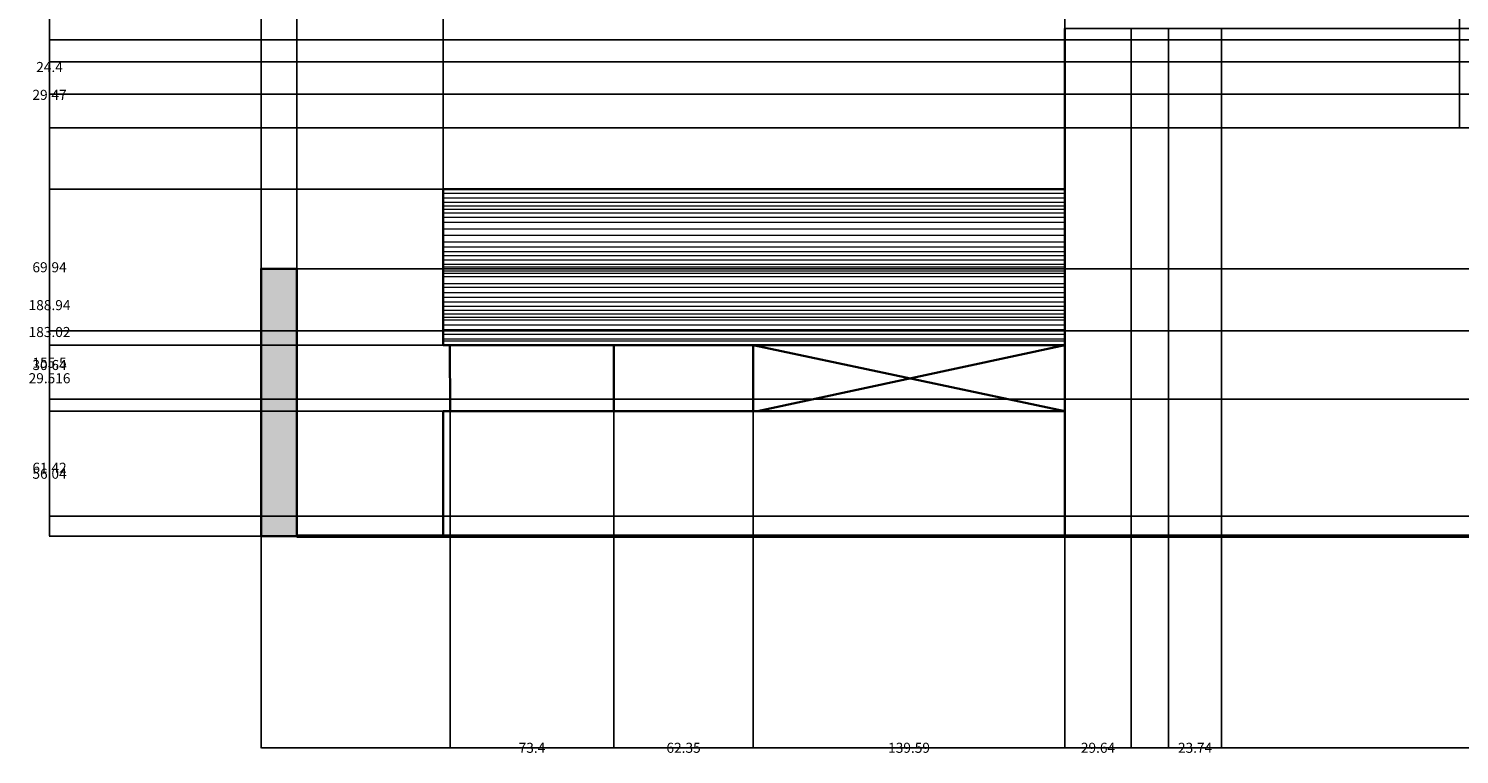
# Model space of a CAD drawing. Units: inches. Extents: x -1308 to 780, y 304 to 1023.
# Tile 1 of 7: x -1308 to -667, y 304 to 629. Entities that reach past the tile are written whole.
import ezdxf

# ---------------------------------------------------------------- set-up
doc = ezdxf.new("R2010")
doc.units = ezdxf.units.IN
doc.header["$MEASUREMENT"] = 0
for name, color, linetype, lineweight in [('A-ANNO-DIMS', 2, 'Continuous', 18), ('A-ELEV', 7, 'Continuous', 35), ('A-ELEV-GRND', 7, 'Continuous', 50), ('A-ELEV-PATT', 8, 'Continuous', 13)]:
    doc.layers.add(name, color=color, linetype=linetype, lineweight=lineweight)
doc.styles.get("Standard").update_dxf_attribs({"font": 'arial.ttf'})
doc.dimstyles.get("Standard").update_dxf_attribs({"dimtxt": 4.5, "dimasz": 0.18, "dimexe": 0.18, "dimexo": 0.0625, "dimgap": 0.09, "dimtad": 0, "dimtih": 1, "dimtoh": 1, "dimdec": 4, "dimzin": 0, "dimdsep": 46, "dimlunit": 4, "dimtxsty": 'Standard', "dimcen": 0.09, "dimadec": 0, "dimazin": 0, "dimtfac": 1, "dimtdec": 4, "dimtofl": 0, "dimtmove": 0, "dimatfit": 3, "dimfxl": 1, "dimtolj": 1, "dimtzin": 0, "dimarcsym": 0})

# ---------------------------------------------------------------- blocks, each defined once
blk = doc.blocks.new('*D1')
at = {"layer": 'A-ANNO-DIMS', "color": 0, "lineweight": -2, "transparency": 16777216}
for p, q in [((-1203.52, 401.95), (-1203.52, 307.09)), ((676.16, 401.95), (676.16, 307.09)), ((-1203.34, 307.27), (-272.9, 307.27)), ((675.98, 307.27), (-254.46, 307.27))]:
    blk.add_line(p, q, dxfattribs=at)
at = {"layer": 'A-ANNO-DIMS', "color": 0, "transparency": 16777216}
for points in [[(-1203.34, 307.3), (-1203.34, 307.24), (-1203.52, 307.27)], [(675.98, 307.3), (675.98, 307.24), (676.16, 307.27)]]:
    blk.add_solid(points, dxfattribs=at)
at = {"layer": 'Defpoints', "color": 0, "transparency": 16777216}
for p in [(-1203.52, 402.02), (676.16, 402.02), (676.16, 307.27)]:
    blk.add_point(p, dxfattribs=at)
at = {"layer": 'A-ANNO-DIMS', "color": 0, "transparency": 16777216, "insert": (-263.68, 307.27), "char_height": 4.5, "attachment_point": 5}
blk.add_mtext('\\A1;1879.7', dxfattribs=at)
blk = doc.blocks.new('*D2')
at = {"layer": 'A-ANNO-DIMS', "color": 0, "lineweight": -2, "transparency": 16777216}
for p, q in [((-1203.52, 521.91), (-1203.52, 1019.77)), ((-1203.34, 1019.59), (-1202.96, 1019.59)), ((-1187.68, 1019.59), (-1188.06, 1019.59)), ((-1187.5, 521.91), (-1187.5, 1019.77))]:
    blk.add_line(p, q, dxfattribs=at)
at = {"layer": 'A-ANNO-DIMS', "color": 0, "transparency": 16777216}
for points in [[(-1203.34, 1019.62), (-1203.34, 1019.56), (-1203.52, 1019.59)], [(-1187.68, 1019.62), (-1187.68, 1019.56), (-1187.5, 1019.59)]]:
    blk.add_solid(points, dxfattribs=at)
at = {"layer": 'Defpoints', "color": 0, "transparency": 16777216}
for p in [(-1187.5, 1019.59), (-1203.52, 521.84), (-1187.5, 521.84)]:
    blk.add_point(p, dxfattribs=at)
at = {"layer": 'A-ANNO-DIMS', "color": 0, "transparency": 16777216, "insert": (-1195.51, 1019.59), "char_height": 4.5, "attachment_point": 5}
blk.add_mtext('\\A1;16.02', dxfattribs=at)
blk = doc.blocks.new('*D3')
at = {"layer": 'A-ANNO-DIMS', "color": 0, "lineweight": -2, "transparency": 16777216}
for p, q in [((-1187.5, 521.91), (-1187.5, 1019.77)), ((-1187.32, 1019.59), (-1162.46, 1019.59)), ((-1122.2, 1019.59), (-1147.07, 1019.59)), ((-1122.02, 557.57), (-1122.02, 1019.77))]:
    blk.add_line(p, q, dxfattribs=at)
at = {"layer": 'A-ANNO-DIMS', "color": 0, "transparency": 16777216}
for points in [[(-1187.32, 1019.62), (-1187.32, 1019.56), (-1187.5, 1019.59)], [(-1122.2, 1019.62), (-1122.2, 1019.56), (-1122.02, 1019.59)]]:
    blk.add_solid(points, dxfattribs=at)
at = {"layer": 'Defpoints', "color": 0, "transparency": 16777216}
for p in [(-1122.02, 1019.59), (-1122.02, 557.51), (-1187.5, 521.84)]:
    blk.add_point(p, dxfattribs=at)
at = {"layer": 'A-ANNO-DIMS', "color": 0, "transparency": 16777216, "insert": (-1154.76, 1019.59), "char_height": 4.5, "attachment_point": 5}
blk.add_mtext('\\A1;65.47', dxfattribs=at)
blk = doc.blocks.new('*D4')
at = {"layer": 'A-ANNO-DIMS', "color": 0, "lineweight": -2, "transparency": 16777216}
for p, q in [((-1122.02, 557.57), (-1122.02, 1019.77)), ((-1121.84, 1019.59), (-990.52, 1019.59)), ((-843.78, 1019.59), (-975.1, 1019.59)), ((-843.6, 557.57), (-843.6, 1019.77))]:
    blk.add_line(p, q, dxfattribs=at)
at = {"layer": 'A-ANNO-DIMS', "color": 0, "transparency": 16777216}
for points in [[(-1121.84, 1019.62), (-1121.84, 1019.56), (-1122.02, 1019.59)], [(-843.78, 1019.62), (-843.78, 1019.56), (-843.6, 1019.59)]]:
    blk.add_solid(points, dxfattribs=at)
at = {"layer": 'Defpoints', "color": 0, "transparency": 16777216}
for p in [(-843.6, 1019.59), (-1122.02, 557.51), (-843.6, 557.51)]:
    blk.add_point(p, dxfattribs=at)
at = {"layer": 'A-ANNO-DIMS', "color": 0, "transparency": 16777216, "insert": (-982.81, 1019.59), "char_height": 4.5, "attachment_point": 5}
blk.add_mtext('\\A1;278.4', dxfattribs=at)
blk = doc.blocks.new('*D5')
at = {"layer": 'A-ANNO-DIMS', "color": 0, "lineweight": -2, "transparency": 16777216}
for p, q in [((-843.6, 402.08), (-843.6, 1019.77)), ((-843.42, 1019.59), (-764.51, 1019.59)), ((-667.13, 1019.59), (-746.04, 1019.59)), ((-666.95, 585.1), (-666.95, 1019.77))]:
    blk.add_line(p, q, dxfattribs=at)
at = {"layer": 'A-ANNO-DIMS', "color": 0, "transparency": 16777216}
for points in [[(-843.42, 1019.62), (-843.42, 1019.56), (-843.6, 1019.59)], [(-667.13, 1019.62), (-667.13, 1019.56), (-666.95, 1019.59)]]:
    blk.add_solid(points, dxfattribs=at)
at = {"layer": 'Defpoints', "color": 0, "transparency": 16777216}
for p in [(-666.95, 1019.59), (-666.95, 585.04), (-843.6, 402.02)]:
    blk.add_point(p, dxfattribs=at)
at = {"layer": 'A-ANNO-DIMS', "color": 0, "transparency": 16777216, "insert": (-755.27, 1019.59), "char_height": 4.5, "attachment_point": 5}
blk.add_mtext('\\A1;176.65', dxfattribs=at)
blk = doc.blocks.new('*D6')
at = {"layer": 'A-ANNO-DIMS', "color": 0, "lineweight": -2, "transparency": 16777216}
for p, q in [((-666.95, 585.1), (-666.95, 1019.77)), ((-666.77, 1019.59), (-519.19, 1019.59)), ((-356.24, 1019.59), (-503.82, 1019.59)), ((-356.06, 585.1), (-356.06, 1019.77))]:
    blk.add_line(p, q, dxfattribs=at)
at = {"layer": 'A-ANNO-DIMS', "color": 0, "transparency": 16777216}
for points in [[(-666.77, 1019.62), (-666.77, 1019.56), (-666.95, 1019.59)], [(-356.24, 1019.62), (-356.24, 1019.56), (-356.06, 1019.59)]]:
    blk.add_solid(points, dxfattribs=at)
at = {"layer": 'Defpoints', "color": 0, "transparency": 16777216}
for p in [(-356.06, 1019.59), (-666.95, 585.04), (-356.06, 585.04)]:
    blk.add_point(p, dxfattribs=at)
at = {"layer": 'A-ANNO-DIMS', "color": 0, "transparency": 16777216, "insert": (-511.5, 1019.59), "char_height": 4.5, "attachment_point": 5}
blk.add_mtext('\\A1;310.9', dxfattribs=at)
blk = doc.blocks.new('*D49')
at = {"layer": 'A-ANNO-DIMS', "color": 0, "lineweight": -2, "transparency": 16777216}
for p, q in [((-843.6, 629.38), (-843.6, 307.09)), ((-813.96, 629.38), (-813.96, 307.09)), ((-843.42, 307.27), (-836.49, 307.27)), ((-814.14, 307.27), (-821.07, 307.27))]:
    blk.add_line(p, q, dxfattribs=at)
at = {"layer": 'A-ANNO-DIMS', "color": 0, "transparency": 16777216}
for points in [[(-843.42, 307.3), (-843.42, 307.24), (-843.6, 307.27)], [(-814.14, 307.3), (-814.14, 307.24), (-813.96, 307.27)]]:
    blk.add_solid(points, dxfattribs=at)
at = {"layer": 'Defpoints', "color": 0, "transparency": 16777216}
for p in [(-843.6, 629.44), (-813.96, 629.44), (-813.96, 307.27)]:
    blk.add_point(p, dxfattribs=at)
at = {"layer": 'A-ANNO-DIMS', "color": 0, "transparency": 16777216, "insert": (-828.78, 307.27), "char_height": 4.5, "attachment_point": 5}
blk.add_mtext('\\A1;29.64', dxfattribs=at)
blk = doc.blocks.new('*D51')
at = {"layer": 'A-ANNO-DIMS', "color": 0, "lineweight": -2, "transparency": 16777216}
for p, q in [((-797.18, 629.38), (-797.18, 307.09)), ((-773.44, 629.38), (-773.44, 307.09)), ((-797, 307.27), (-793.02, 307.27)), ((-773.62, 307.27), (-777.6, 307.27))]:
    blk.add_line(p, q, dxfattribs=at)
at = {"layer": 'A-ANNO-DIMS', "color": 0, "transparency": 16777216}
for points in [[(-797, 307.3), (-797, 307.24), (-797.18, 307.27)], [(-773.62, 307.3), (-773.62, 307.24), (-773.44, 307.27)]]:
    blk.add_solid(points, dxfattribs=at)
at = {"layer": 'Defpoints', "color": 0, "transparency": 16777216}
for p in [(-797.18, 629.44), (-773.44, 629.44), (-773.44, 307.27)]:
    blk.add_point(p, dxfattribs=at)
at = {"layer": 'A-ANNO-DIMS', "color": 0, "transparency": 16777216, "insert": (-785.31, 307.27), "char_height": 4.5, "attachment_point": 5}
blk.add_mtext('\\A1;23.74', dxfattribs=at)
blk = doc.blocks.new('*D52')
at = {"layer": 'A-ANNO-DIMS', "color": 0, "lineweight": -2, "transparency": 16777216}
for p, q in [((-1118.94, 457.99), (-1118.94, 307.09)), ((-1045.54, 457.99), (-1045.54, 307.09)), ((-1118.76, 307.27), (-1088.14, 307.27)), ((-1045.72, 307.27), (-1076.33, 307.27))]:
    blk.add_line(p, q, dxfattribs=at)
at = {"layer": 'A-ANNO-DIMS', "color": 0, "transparency": 16777216}
for points in [[(-1118.76, 307.3), (-1118.76, 307.24), (-1118.94, 307.27)], [(-1045.72, 307.3), (-1045.72, 307.24), (-1045.54, 307.27)]]:
    blk.add_solid(points, dxfattribs=at)
at = {"layer": 'Defpoints', "color": 0, "transparency": 16777216}
for p in [(-1118.94, 458.06), (-1045.54, 458.06), (-1045.54, 307.27)]:
    blk.add_point(p, dxfattribs=at)
at = {"layer": 'A-ANNO-DIMS', "color": 0, "transparency": 16777216, "insert": (-1082.24, 307.27), "char_height": 4.5, "attachment_point": 5}
blk.add_mtext('\\A1;73.4', dxfattribs=at)
blk = doc.blocks.new('*D53')
at = {"layer": 'A-ANNO-DIMS', "color": 0, "lineweight": -2, "transparency": 16777216}
for p, q in [((-1045.54, 457.99), (-1045.54, 307.09)), ((-983.18, 457.99), (-983.18, 307.09)), ((-1045.36, 307.27), (-1022.07, 307.27)), ((-983.36, 307.27), (-1006.65, 307.27))]:
    blk.add_line(p, q, dxfattribs=at)
at = {"layer": 'A-ANNO-DIMS', "color": 0, "transparency": 16777216}
for points in [[(-1045.36, 307.3), (-1045.36, 307.24), (-1045.54, 307.27)], [(-983.36, 307.3), (-983.36, 307.24), (-983.18, 307.27)]]:
    blk.add_solid(points, dxfattribs=at)
at = {"layer": 'Defpoints', "color": 0, "transparency": 16777216}
for p in [(-1045.54, 458.06), (-983.18, 458.06), (-983.18, 307.27)]:
    blk.add_point(p, dxfattribs=at)
at = {"layer": 'A-ANNO-DIMS', "color": 0, "transparency": 16777216, "insert": (-1014.36, 307.27), "char_height": 4.5, "attachment_point": 5}
blk.add_mtext('\\A1;62.35', dxfattribs=at)
blk = doc.blocks.new('*D54')
at = {"layer": 'A-ANNO-DIMS', "color": 0, "lineweight": -2, "transparency": 16777216}
for p, q in [((-983.18, 457.99), (-983.18, 307.09)), ((-843.6, 457.99), (-843.6, 307.09)), ((-983, 307.27), (-922.62, 307.27)), ((-843.78, 307.27), (-904.17, 307.27))]:
    blk.add_line(p, q, dxfattribs=at)
at = {"layer": 'A-ANNO-DIMS', "color": 0, "transparency": 16777216}
for points in [[(-983, 307.3), (-983, 307.24), (-983.18, 307.27)], [(-843.78, 307.3), (-843.78, 307.24), (-843.6, 307.27)]]:
    blk.add_solid(points, dxfattribs=at)
at = {"layer": 'Defpoints', "color": 0, "transparency": 16777216}
for p in [(-983.18, 458.06), (-843.6, 458.06), (-843.6, 307.27)]:
    blk.add_point(p, dxfattribs=at)
at = {"layer": 'A-ANNO-DIMS', "color": 0, "transparency": 16777216, "insert": (-913.39, 307.27), "char_height": 4.5, "attachment_point": 5}
blk.add_mtext('\\A1;139.59', dxfattribs=at)
blk = doc.blocks.new('*D57')
at = {"layer": 'A-ANNO-DIMS', "color": 0, "lineweight": -2, "transparency": 16777216}
for p, q in [((-628.74, 924.84), (-1298.45, 924.84)), ((-1298.27, 924.66), (-1298.27, 665.82)), ((-1298.27, 402.2), (-1298.27, 661.04)), ((-1203.58, 402.02), (-1298.45, 402.02))]:
    blk.add_line(p, q, dxfattribs=at)
at = {"layer": 'A-ANNO-DIMS', "color": 0, "transparency": 16777216}
for points in [[(-1298.3, 924.66), (-1298.24, 924.66), (-1298.27, 924.84)], [(-1298.3, 402.2), (-1298.24, 402.2), (-1298.27, 402.02)]]:
    blk.add_solid(points, dxfattribs=at)
at = {"layer": 'Defpoints', "color": 0, "transparency": 16777216}
for p in [(-1298.27, 924.84), (-628.68, 924.84), (-1203.52, 402.02)]:
    blk.add_point(p, dxfattribs=at)
at = {"layer": 'A-ANNO-DIMS', "color": 0, "transparency": 16777216, "insert": (-1298.27, 663.43), "char_height": 4.5, "attachment_point": 5}
blk.add_mtext('\\A1;522.8', dxfattribs=at)
blk = doc.blocks.new('*D58')
at = {"layer": 'A-ANNO-DIMS', "color": 0, "lineweight": -2, "transparency": 16777216}
for p, q in [((-1187.44, 521.84), (771.09, 521.84)), ((770.91, 521.66), (770.91, 464.32)), ((770.91, 402.2), (770.91, 459.54)), ((-1187.44, 402.02), (771.09, 402.02))]:
    blk.add_line(p, q, dxfattribs=at)
at = {"layer": 'A-ANNO-DIMS', "color": 0, "transparency": 16777216}
for points in [[(770.88, 521.66), (770.94, 521.66), (770.91, 521.84)], [(770.88, 402.2), (770.94, 402.2), (770.91, 402.02)]]:
    blk.add_solid(points, dxfattribs=at)
at = {"layer": 'Defpoints', "color": 0, "transparency": 16777216}
for p in [(-1187.5, 521.84), (770.91, 521.84), (-1187.5, 402.02)]:
    blk.add_point(p, dxfattribs=at)
at = {"layer": 'A-ANNO-DIMS', "color": 0, "transparency": 16777216, "insert": (770.91, 461.93), "char_height": 4.5, "attachment_point": 5}
blk.add_mtext('\\A1;119.83', dxfattribs=at)
blk = doc.blocks.new('*D59')
at = {"layer": 'A-ANNO-DIMS', "color": 0, "lineweight": -2, "transparency": 16777216}
for p, q in [((-1122.09, 557.51), (-1298.45, 557.51)), ((-1298.27, 557.33), (-1298.27, 482.15)), ((-1298.27, 402.2), (-1298.27, 477.38)), ((-1122.09, 402.02), (-1298.45, 402.02))]:
    blk.add_line(p, q, dxfattribs=at)
at = {"layer": 'A-ANNO-DIMS', "color": 0, "transparency": 16777216}
for points in [[(-1298.3, 557.33), (-1298.24, 557.33), (-1298.27, 557.51)], [(-1298.3, 402.2), (-1298.24, 402.2), (-1298.27, 402.02)]]:
    blk.add_solid(points, dxfattribs=at)
at = {"layer": 'Defpoints', "color": 0, "transparency": 16777216}
for p in [(-1298.27, 557.51), (-1122.02, 557.51), (-1122.02, 402.02)]:
    blk.add_point(p, dxfattribs=at)
at = {"layer": 'A-ANNO-DIMS', "color": 0, "transparency": 16777216, "insert": (-1298.27, 479.76), "char_height": 4.5, "attachment_point": 5}
blk.add_mtext('\\A1;155.5', dxfattribs=at)
blk = doc.blocks.new('*D60')
at = {"layer": 'A-ANNO-DIMS', "color": 0, "lineweight": -2, "transparency": 16777216}
for p, q in [((-843.66, 458.06), (-1298.45, 458.06)), ((-1298.27, 457.88), (-1298.27, 432.42)), ((-1298.27, 402.2), (-1298.27, 427.65)), ((-843.66, 402.02), (-1298.45, 402.02))]:
    blk.add_line(p, q, dxfattribs=at)
at = {"layer": 'A-ANNO-DIMS', "color": 0, "transparency": 16777216}
for points in [[(-1298.3, 457.88), (-1298.24, 457.88), (-1298.27, 458.06)], [(-1298.3, 402.2), (-1298.24, 402.2), (-1298.27, 402.02)]]:
    blk.add_solid(points, dxfattribs=at)
at = {"layer": 'Defpoints', "color": 0, "transparency": 16777216}
for p in [(-1298.27, 458.06), (-843.6, 458.06), (-843.6, 402.02)]:
    blk.add_point(p, dxfattribs=at)
at = {"layer": 'A-ANNO-DIMS', "color": 0, "transparency": 16777216, "insert": (-1298.27, 430.04), "char_height": 4.5, "attachment_point": 5}
blk.add_mtext('\\A1;56.04', dxfattribs=at)
blk = doc.blocks.new('*D61')
at = {"layer": 'A-ANNO-DIMS', "color": 0, "lineweight": -2, "transparency": 16777216}
for p, q in [((-843.66, 487.57), (-1298.45, 487.57)), ((-1298.27, 487.39), (-1298.27, 475.2)), ((-1298.27, 458.24), (-1298.27, 470.43)), ((-843.66, 458.06), (-1298.45, 458.06))]:
    blk.add_line(p, q, dxfattribs=at)
at = {"layer": 'A-ANNO-DIMS', "color": 0, "transparency": 16777216}
for points in [[(-1298.3, 487.39), (-1298.24, 487.39), (-1298.27, 487.57)], [(-1298.3, 458.24), (-1298.24, 458.24), (-1298.27, 458.06)]]:
    blk.add_solid(points, dxfattribs=at)
at = {"layer": 'Defpoints', "color": 0, "transparency": 16777216}
for p in [(-1298.27, 487.57), (-843.6, 487.57), (-843.6, 458.06)]:
    blk.add_point(p, dxfattribs=at)
at = {"layer": 'A-ANNO-DIMS', "color": 0, "transparency": 16777216, "insert": (-1298.27, 472.82), "char_height": 4.5, "attachment_point": 5}
blk.add_mtext('\\A1;29.516', dxfattribs=at)
blk = doc.blocks.new('*D62')
at = {"layer": 'A-ANNO-DIMS', "color": 0, "lineweight": -2, "transparency": 16777216}
for p, q in [((-843.66, 557.51), (-1298.45, 557.51)), ((-1298.27, 557.33), (-1298.27, 524.93)), ((-1298.27, 487.75), (-1298.27, 520.15)), ((-843.66, 487.57), (-1298.45, 487.57))]:
    blk.add_line(p, q, dxfattribs=at)
at = {"layer": 'A-ANNO-DIMS', "color": 0, "transparency": 16777216}
for points in [[(-1298.3, 557.33), (-1298.24, 557.33), (-1298.27, 557.51)], [(-1298.3, 487.75), (-1298.24, 487.75), (-1298.27, 487.57)]]:
    blk.add_solid(points, dxfattribs=at)
at = {"layer": 'Defpoints', "color": 0, "transparency": 16777216}
for p in [(-1298.27, 557.51), (-843.6, 557.51), (-843.6, 487.57)]:
    blk.add_point(p, dxfattribs=at)
at = {"layer": 'A-ANNO-DIMS', "color": 0, "transparency": 16777216, "insert": (-1298.27, 522.54), "char_height": 4.5, "attachment_point": 5}
blk.add_mtext('\\A1;69.94', dxfattribs=at)
blk = doc.blocks.new('*D63')
at = {"layer": 'A-ANNO-DIMS', "color": 0, "lineweight": -2, "transparency": 16777216}
for p, q in [((-843.54, 629.44), (771.09, 629.44)), ((770.91, 629.26), (770.91, 518.12)), ((770.91, 402.2), (770.91, 513.34)), ((-843.54, 402.02), (771.09, 402.02))]:
    blk.add_line(p, q, dxfattribs=at)
at = {"layer": 'A-ANNO-DIMS', "color": 0, "transparency": 16777216}
for points in [[(770.88, 629.26), (770.94, 629.26), (770.91, 629.44)], [(770.88, 402.2), (770.94, 402.2), (770.91, 402.02)]]:
    blk.add_solid(points, dxfattribs=at)
at = {"layer": 'Defpoints', "color": 0, "transparency": 16777216}
for p in [(-843.6, 629.44), (770.91, 629.44), (-843.6, 402.02)]:
    blk.add_point(p, dxfattribs=at)
at = {"layer": 'A-ANNO-DIMS', "color": 0, "transparency": 16777216, "insert": (770.91, 515.73), "char_height": 4.5, "attachment_point": 5}
blk.add_mtext('\\A1;227.43', dxfattribs=at)
blk = doc.blocks.new('*D64')
at = {"layer": 'A-ANNO-DIMS', "color": 0, "lineweight": -2, "transparency": 16777216}
for p, q in [((-843.54, 704.09), (771.09, 704.09)), ((770.91, 703.91), (770.91, 669.15)), ((770.91, 629.62), (770.91, 664.38)), ((-843.54, 629.44), (771.09, 629.44))]:
    blk.add_line(p, q, dxfattribs=at)
at = {"layer": 'A-ANNO-DIMS', "color": 0, "transparency": 16777216}
for points in [[(770.88, 703.91), (770.94, 703.91), (770.91, 704.09)], [(770.88, 629.62), (770.94, 629.62), (770.91, 629.44)]]:
    blk.add_solid(points, dxfattribs=at)
at = {"layer": 'Defpoints', "color": 0, "transparency": 16777216}
for p in [(-843.6, 704.09), (770.91, 704.09), (-843.6, 629.44)]:
    blk.add_point(p, dxfattribs=at)
at = {"layer": 'A-ANNO-DIMS', "color": 0, "transparency": 16777216, "insert": (770.91, 666.76), "char_height": 4.5, "attachment_point": 5}
blk.add_mtext('\\A1;74.64', dxfattribs=at)
blk = doc.blocks.new('*D66')
at = {"layer": 'A-ANNO-DIMS', "color": 0, "lineweight": -2, "transparency": 16777216}
for p, q in [((-667.01, 585.04), (-1298.45, 585.04)), ((-1298.27, 584.86), (-1298.27, 495.92)), ((-1298.27, 402.2), (-1298.27, 491.14)), ((-667.01, 402.02), (-1298.45, 402.02))]:
    blk.add_line(p, q, dxfattribs=at)
at = {"layer": 'A-ANNO-DIMS', "color": 0, "transparency": 16777216}
for points in [[(-1298.3, 584.86), (-1298.24, 584.86), (-1298.27, 585.04)], [(-1298.3, 402.2), (-1298.24, 402.2), (-1298.27, 402.02)]]:
    blk.add_solid(points, dxfattribs=at)
at = {"layer": 'Defpoints', "color": 0, "transparency": 16777216}
for p in [(-1298.27, 585.04), (-666.95, 585.04), (-666.95, 402.02)]:
    blk.add_point(p, dxfattribs=at)
at = {"layer": 'A-ANNO-DIMS', "color": 0, "transparency": 16777216, "insert": (-1298.27, 493.53), "char_height": 4.5, "attachment_point": 5}
blk.add_mtext('\\A1;183.02', dxfattribs=at)
blk = doc.blocks.new('*D67')
at = {"layer": 'A-ANNO-DIMS', "color": 0, "lineweight": -2, "transparency": 16777216}
for p, q in [((-271.41, 600.04), (-1298.45, 600.04)), ((-1298.27, 599.86), (-1298.27, 507.96)), ((-1298.27, 411.28), (-1298.27, 503.18)), ((-271.41, 411.1), (-1298.45, 411.1))]:
    blk.add_line(p, q, dxfattribs=at)
at = {"layer": 'A-ANNO-DIMS', "color": 0, "transparency": 16777216}
for points in [[(-1298.3, 599.86), (-1298.24, 599.86), (-1298.27, 600.04)], [(-1298.3, 411.28), (-1298.24, 411.28), (-1298.27, 411.1)]]:
    blk.add_solid(points, dxfattribs=at)
at = {"layer": 'Defpoints', "color": 0, "transparency": 16777216}
for p in [(-1298.27, 600.04), (-271.35, 600.04), (-271.35, 411.1)]:
    blk.add_point(p, dxfattribs=at)
at = {"layer": 'A-ANNO-DIMS', "color": 0, "transparency": 16777216, "insert": (-1298.27, 505.57), "char_height": 4.5, "attachment_point": 5}
blk.add_mtext('\\A1;188.94', dxfattribs=at)
blk = doc.blocks.new('*D68')
at = {"layer": 'A-ANNO-DIMS', "color": 0, "lineweight": -2, "transparency": 16777216}
for p, q in [((-271.41, 624.44), (-1298.45, 624.44)), ((-1298.27, 624.26), (-1298.27, 614.59)), ((-1298.27, 600.22), (-1298.27, 609.89)), ((-271.41, 600.04), (-1298.45, 600.04))]:
    blk.add_line(p, q, dxfattribs=at)
at = {"layer": 'A-ANNO-DIMS', "color": 0, "transparency": 16777216}
for points in [[(-1298.3, 624.26), (-1298.24, 624.26), (-1298.27, 624.44)], [(-1298.3, 600.22), (-1298.24, 600.22), (-1298.27, 600.04)]]:
    blk.add_solid(points, dxfattribs=at)
at = {"layer": 'Defpoints', "color": 0, "transparency": 16777216}
for p in [(-1298.27, 624.44), (-271.35, 624.44), (-271.35, 600.04)]:
    blk.add_point(p, dxfattribs=at)
at = {"layer": 'A-ANNO-DIMS', "color": 0, "transparency": 16777216, "insert": (-1298.27, 612.24), "char_height": 4.5, "attachment_point": 5}
blk.add_mtext('\\A1;24.4', dxfattribs=at)
blk = doc.blocks.new('*D69')
at = {"layer": 'A-ANNO-DIMS', "color": 0, "lineweight": -2, "transparency": 16777216}
for p, q in [((-271.41, 739.03), (-1298.45, 739.03)), ((-1298.27, 738.85), (-1298.27, 684.12)), ((-1298.27, 624.62), (-1298.27, 679.35)), ((-271.41, 624.44), (-1298.45, 624.44))]:
    blk.add_line(p, q, dxfattribs=at)
at = {"layer": 'A-ANNO-DIMS', "color": 0, "transparency": 16777216}
for points in [[(-1298.3, 738.85), (-1298.24, 738.85), (-1298.27, 739.03)], [(-1298.3, 624.62), (-1298.24, 624.62), (-1298.27, 624.44)]]:
    blk.add_solid(points, dxfattribs=at)
at = {"layer": 'Defpoints', "color": 0, "transparency": 16777216}
for p in [(-1298.27, 739.03), (-271.35, 739.03), (-271.35, 624.44)]:
    blk.add_point(p, dxfattribs=at)
at = {"layer": 'A-ANNO-DIMS', "color": 0, "transparency": 16777216, "insert": (-1298.27, 681.73), "char_height": 4.5, "attachment_point": 5}
blk.add_mtext('\\A1;114.58', dxfattribs=at)
blk = doc.blocks.new('*D79')
at = {"layer": 'A-ANNO-DIMS', "color": 0, "lineweight": -2, "transparency": 16777216}
for p, q in [((310.7, 463.43), (-1298.45, 463.43)), ((-1298.27, 463.25), (-1298.27, 435.11)), ((-1298.27, 402.2), (-1298.27, 430.34)), ((296.47, 402.02), (-1298.45, 402.02))]:
    blk.add_line(p, q, dxfattribs=at)
at = {"layer": 'A-ANNO-DIMS', "color": 0, "transparency": 16777216}
for points in [[(-1298.3, 463.25), (-1298.24, 463.25), (-1298.27, 463.43)], [(-1298.3, 402.2), (-1298.24, 402.2), (-1298.27, 402.02)]]:
    blk.add_solid(points, dxfattribs=at)
at = {"layer": 'Defpoints', "color": 0, "transparency": 16777216}
for p in [(-1298.27, 463.43), (310.77, 463.43), (296.53, 402.02)]:
    blk.add_point(p, dxfattribs=at)
at = {"layer": 'A-ANNO-DIMS', "color": 0, "transparency": 16777216, "insert": (-1298.27, 432.72), "char_height": 4.5, "attachment_point": 5}
blk.add_mtext('\\A1;61.42', dxfattribs=at)
blk = doc.blocks.new('*D80')
at = {"layer": 'A-ANNO-DIMS', "color": 0, "lineweight": -2, "transparency": 16777216}
for p, q in [((308.7, 494.07), (-1298.45, 494.07)), ((-1298.27, 493.89), (-1298.27, 481.14)), ((-1298.27, 463.61), (-1298.27, 476.36)), ((310.7, 463.43), (-1298.45, 463.43))]:
    blk.add_line(p, q, dxfattribs=at)
at = {"layer": 'A-ANNO-DIMS', "color": 0, "transparency": 16777216}
for points in [[(-1298.3, 493.89), (-1298.24, 493.89), (-1298.27, 494.07)], [(-1298.3, 463.61), (-1298.24, 463.61), (-1298.27, 463.43)]]:
    blk.add_solid(points, dxfattribs=at)
at = {"layer": 'Defpoints', "color": 0, "transparency": 16777216}
for p in [(-1298.27, 494.07), (308.77, 494.07), (310.77, 463.43)]:
    blk.add_point(p, dxfattribs=at)
at = {"layer": 'A-ANNO-DIMS', "color": 0, "transparency": 16777216, "insert": (-1298.27, 478.75), "char_height": 4.5, "attachment_point": 5}
blk.add_mtext('\\A1;30.64', dxfattribs=at)
blk = doc.blocks.new('*D81')
at = {"layer": 'A-ANNO-DIMS', "color": 0, "lineweight": -2, "transparency": 16777216}
for p, q in [((-25.92, 614.51), (-1298.45, 614.51)), ((-1298.27, 614.33), (-1298.27, 602.16)), ((-1298.27, 585.22), (-1298.27, 597.39)), ((-59.22, 585.04), (-1298.45, 585.04))]:
    blk.add_line(p, q, dxfattribs=at)
at = {"layer": 'A-ANNO-DIMS', "color": 0, "transparency": 16777216}
for points in [[(-1298.3, 614.33), (-1298.24, 614.33), (-1298.27, 614.51)], [(-1298.3, 585.22), (-1298.24, 585.22), (-1298.27, 585.04)]]:
    blk.add_solid(points, dxfattribs=at)
at = {"layer": 'Defpoints', "color": 0, "transparency": 16777216}
for p in [(-1298.27, 614.51), (-25.86, 614.51), (-59.16, 585.04)]:
    blk.add_point(p, dxfattribs=at)
at = {"layer": 'A-ANNO-DIMS', "color": 0, "transparency": 16777216, "insert": (-1298.27, 599.77), "char_height": 4.5, "attachment_point": 5}
blk.add_mtext('\\A1;29.47', dxfattribs=at)
blk = doc.blocks.new('*D82')
at = {"layer": 'A-ANNO-DIMS', "color": 0, "lineweight": -2, "transparency": 16777216}
for p, q in [((-25.92, 709.46), (-1298.45, 709.46)), ((-1298.27, 709.28), (-1298.27, 664.37)), ((-1298.27, 614.69), (-1298.27, 659.6)), ((-25.92, 614.51), (-1298.45, 614.51))]:
    blk.add_line(p, q, dxfattribs=at)
at = {"layer": 'A-ANNO-DIMS', "color": 0, "transparency": 16777216}
for points in [[(-1298.3, 709.28), (-1298.24, 709.28), (-1298.27, 709.46)], [(-1298.3, 614.69), (-1298.24, 614.69), (-1298.27, 614.51)]]:
    blk.add_solid(points, dxfattribs=at)
at = {"layer": 'Defpoints', "color": 0, "transparency": 16777216}
for p in [(-1298.27, 709.46), (-25.86, 709.46), (-25.86, 614.51)]:
    blk.add_point(p, dxfattribs=at)
at = {"layer": 'A-ANNO-DIMS', "color": 0, "transparency": 16777216, "insert": (-1298.27, 661.98), "char_height": 4.5, "attachment_point": 5}
blk.add_mtext('\\A1;94.95', dxfattribs=at)

msp = doc.modelspace()

# ---------------------------------------------------------------- hatches: boundary and pattern name
at = {"layer": 'A-ELEV-PATT'}
h = msp.add_hatch(color=256, dxfattribs=at)
h.dxf.hatch_style = 1
h.paths.add_polyline_path([(-1187.498, 521.8442), (-1203.518, 521.8442), (-1203.518, 402.0158), (-1187.498, 402.0158)])

# ---------------------------------------------------------------- linework, layer by layer
at = {"layer": 'A-ELEV'}
for p, q in [((-843.5988, 402.0158), (-843.5988, 629.4421)), ((-843.5988, 557.5099), (-1122.0239, 557.5099)), ((-1122.0239, 557.5099), (-1122.0239, 487.5731)), ((-1122.0239, 487.5731), (-843.5988, 487.5731)), ((-1119.0414, 487.5731), (-1118.9378, 458.0575)), ((-1045.536, 487.5731), (-1045.536, 458.0575)), ((-983.1843, 487.5731), (-983.1843, 458.0575)), ((-983.1843, 487.5731), (-843.5988, 458.0575)), ((-843.5988, 487.5731), (-981.2014, 458.0575)), ((-1118.804, 458.0575), (-1122.0239, 458.0575)), ((-1122.0239, 458.0575), (-1122.0239, 402.0158)), ((-1118.804, 458.0575), (-843.5988, 458.0575))]:
    msp.add_line(p, q, dxfattribs=at)
msp.add_lwpolyline([(-1187.498, 402.0158), (-1203.518, 402.0158), (-1203.518, 521.8442), (-1187.498, 521.8442)], close=True, dxfattribs=at)
at = {"layer": 'A-ELEV-GRND'}
for p, q in [((-843.5988, 402.0158), (-1187.498, 402.0158)), ((-725.0987, 402.0158), (-843.5988, 402.0158)), ((-608.7933, 402.0158), (-725.0987, 402.0158))]:
    msp.add_line(p, q, dxfattribs=at)
at = {"layer": 'A-ELEV-PATT'}
for p, q in [((-843.5988, 555.5099), (-1122.0239, 555.5099)), ((-843.5988, 553.5099), (-1122.0239, 553.5099)), ((-843.5988, 551.5099), (-1122.0239, 551.5099)), ((-843.5988, 549.8438), (-1122.0239, 549.8438)), ((-843.5988, 548.4036), (-1122.0239, 548.4036)), ((-843.5988, 546.7276), (-1122.0239, 546.7276)), ((-843.5988, 544.8654), (-1122.0239, 544.8654)), ((-843.5988, 542.6573), (-1122.0239, 542.6573)), ((-843.5988, 539.6162), (-1122.0239, 539.6162)), ((-843.5988, 536.7119), (-1122.0239, 536.7119)), ((-843.5988, 533.759), (-1122.0239, 533.759)), ((-843.5988, 531.5509), (-1122.0239, 531.5509)), ((-843.5988, 529.4408), (-1122.0239, 529.4408)), ((-843.5988, 527.6052), (-1122.0239, 527.6052)), ((-843.5988, 525.7696), (-1122.0239, 525.7696)), ((-843.5988, 523.6946), (-1122.0239, 523.6946)), ((-843.5988, 522.5415), (-1122.0239, 522.5415)), ((-843.9547, 520.7682), (-1122.0239, 520.7682)), ((-843.5988, 519.663), (-1122.0239, 519.663)), ((-843.5988, 515.1405), (-1122.0239, 515.1405)), ((-843.5988, 513.4113), (-1122.0239, 513.4113)), ((-843.5559, 518.2797), (-1121.9811, 518.2797)), ((-843.5988, 511.1188), (-1122.0239, 511.1188)), ((-843.5988, 508.9639), (-1122.0239, 508.9639)), ((-843.5988, 506.8499), (-1122.0239, 506.8499)), ((-843.5988, 504.8813), (-1122.0239, 504.8813)), ((-843.5988, 503.1521), (-1122.0239, 503.1521)), ((-843.5988, 501.4495), (-1122.0239, 501.4495)), ((-843.5988, 499.9598), (-1122.0239, 499.9598)), ((-843.5988, 498.8424), (-1122.0239, 498.8424)), ((-843.5988, 496.528), (-1122.0239, 496.528)), ((-843.5988, 494.5694), (-1122.0239, 494.5694)), ((-843.5988, 492.3879), (-1122.0239, 492.3879)), ((-843.5988, 490.3129), (-1122.0239, 490.3129)), ((-843.5988, 489.3552), (-1122.0239, 489.3552))]:
    msp.add_line(p, q, dxfattribs=at)

# ---------------------------------------------------------------- dimensions: what is measured, and where the dimension line sits
at = {"layer": 'A-ANNO-DIMS'}
for base, p1, p2, override, picture, middle in [((-1187.498, 1019.5921), (-1203.518, 521.8442), (-1187.498, 521.8442), {"dimdec": 2, "dimlfac": 1, "dimrnd": 0, "dimzin": 0, "dimdsep": 46, "dimlunit": 2}, '*D2', (-1195.508, 1019.5921)), ((-1122.0239, 1019.5921), (-1187.498, 521.8442), (-1122.0239, 557.5099), {"dimdec": 2, "dimlfac": 1, "dimrnd": 0, "dimzin": 0, "dimdsep": 46, "dimlunit": 2}, '*D3', (-1154.761, 1019.5921)), ((-843.5988, 1019.5921), (-1122.0239, 557.5099), (-843.5988, 557.5099), {"dimdec": 1, "dimlfac": 1, "dimrnd": 0, "dimzin": 0, "dimdsep": 46, "dimlunit": 2}, '*D4', (-982.8114, 1019.5921)), ((-666.946, 1019.5921), (-843.5988, 402.0158), (-666.946, 585.0385), {"dimdec": 2, "dimlfac": 1, "dimrnd": 0, "dimzin": 0, "dimdsep": 46, "dimlunit": 2}, '*D5', (-755.2724, 1019.5921)), ((-356.0562, 1019.5921), (-666.946, 585.0385), (-356.0562, 585.0385), {"dimdec": 1, "dimlfac": 1, "dimrnd": 0, "dimzin": 0, "dimdsep": 46, "dimlunit": 2}, '*D6', (-511.5011, 1019.5921)), ((-813.9606, 307.2658), (-843.5988, 629.4421), (-813.9606, 629.4421), {"dimdec": 2, "dimlfac": 1, "dimrnd": 0, "dimzin": 0, "dimdsep": 46, "dimlunit": 2}, '*D49', (-828.7797, 307.2658)), ((-773.441, 307.2658), (-797.1797, 629.4421), (-773.441, 629.4421), {"dimdec": 2, "dimlfac": 1, "dimrnd": 0, "dimzin": 0, "dimdsep": 46, "dimlunit": 2}, '*D51', (-785.3103, 307.2658)), ((-1045.536, 307.2658), (-1118.9378, 458.0575), (-1045.536, 458.0575), {"dimdec": 1, "dimlfac": 1, "dimrnd": 0, "dimzin": 0, "dimdsep": 46, "dimlunit": 2}, '*D52', (-1082.2369, 307.2658)), ((-983.1843, 307.2658), (-1045.536, 458.0575), (-983.1843, 458.0575), {"dimdec": 2, "dimlfac": 1, "dimrnd": 0, "dimzin": 0, "dimdsep": 46, "dimlunit": 2}, '*D53', (-1014.3601, 307.2658)), ((-843.5988, 307.2658), (-983.1843, 458.0575), (-843.5988, 458.0575), {"dimdec": 2, "dimlfac": 1, "dimrnd": 0, "dimzin": 0, "dimdsep": 46, "dimlunit": 2}, '*D54', (-913.3915, 307.2658)), ((676.1576, 307.2658), (-1203.518, 402.0158), (676.1576, 402.0158), {"dimdec": 1, "dimlfac": 1, "dimrnd": 0, "dimzin": 0, "dimdsep": 46, "dimlunit": 2}, '*D1', (-263.6802, 307.2658))]:
    dim = msp.add_linear_dim(base=base, p1=p1, p2=p2, dimstyle='Standard', override=override, dxfattribs=at)
    dim.commit()
    dim.dimension.update_dxf_attribs({"geometry": picture, "text_midpoint": middle})
for base, p1, p2, override, picture, middle in [((-1298.268, 924.8421), (-1203.518, 402.0158), (-628.6809, 924.8421), {"dimdec": 1, "dimlfac": 1, "dimrnd": 0, "dimzin": 0, "dimdsep": 46, "dimlunit": 2}, '*D57', (-1298.268, 663.429)), ((-1298.268, 739.0259), (-271.346, 624.4429), (-271.346, 739.0259), {"dimdec": 2, "dimlfac": 1, "dimrnd": 0, "dimzin": 0, "dimdsep": 46, "dimlunit": 2}, '*D69', (-1298.268, 681.7344)), ((-1298.268, 709.4602), (-25.8575, 614.5069), (-25.8575, 709.4602), {"dimdec": 2, "dimlfac": 1, "dimrnd": 0, "dimzin": 0, "dimdsep": 46, "dimlunit": 2}, '*D82', (-1298.268, 661.9835)), ((770.9076, 704.0857), (-843.5988, 629.4421), (-843.5988, 704.0857), {"dimdec": 2, "dimlfac": 1, "dimrnd": 0, "dimzin": 0, "dimdsep": 46, "dimlunit": 2}, '*D64', (770.9076, 666.7639)), ((770.9076, 629.4421), (-843.5988, 402.0158), (-843.5988, 629.4421), {"dimdec": 2, "dimlfac": 1, "dimrnd": 0, "dimzin": 0, "dimdsep": 46, "dimlunit": 2}, '*D63', (770.9076, 515.729)), ((-1298.268, 624.4429), (-271.346, 600.0434), (-271.346, 624.4429), {"dimdec": 1, "dimlfac": 1, "dimrnd": 0, "dimzin": 0, "dimdsep": 46, "dimlunit": 2}, '*D68', (-1298.268, 612.2432)), ((-1298.268, 614.5069), (-59.1597, 585.0385), (-25.8575, 614.5069), {"dimdec": 2, "dimlfac": 1, "dimrnd": 0, "dimzin": 0, "dimdsep": 46, "dimlunit": 2}, '*D81', (-1298.268, 599.7727)), ((-1298.268, 600.0434), (-271.346, 411.1006), (-271.346, 600.0434), {"dimdec": 2, "dimlfac": 1, "dimrnd": 0, "dimzin": 0, "dimdsep": 46, "dimlunit": 2}, '*D67', (-1298.268, 505.572)), ((-1298.268, 585.0385), (-666.946, 402.0158), (-666.946, 585.0385), {"dimdec": 2, "dimlfac": 1, "dimrnd": 0, "dimzin": 0, "dimdsep": 46, "dimlunit": 2}, '*D66', (-1298.268, 493.5272)), ((-1298.268, 557.5099), (-1122.0239, 402.0158), (-1122.0239, 557.5099), {"dimdec": 1, "dimlfac": 1, "dimrnd": 0, "dimzin": 0, "dimdsep": 46, "dimlunit": 2}, '*D59', (-1298.268, 479.7629)), ((-1298.268, 557.5099), (-843.5988, 487.5731), (-843.5988, 557.5099), {"dimdec": 2, "dimlfac": 1, "dimrnd": 0, "dimzin": 0, "dimdsep": 46, "dimlunit": 2}, '*D62', (-1298.268, 522.5415)), ((770.9076, 521.8442), (-1187.498, 402.0158), (-1187.498, 521.8442), {"dimdec": 2, "dimlfac": 1, "dimrnd": 0, "dimzin": 0, "dimdsep": 46, "dimlunit": 2}, '*D58', (770.9076, 461.93)), ((-1298.268, 494.0703), (310.7651, 463.4331), (308.7651, 494.0703), {"dimdec": 2, "dimlfac": 1, "dimrnd": 0, "dimzin": 0, "dimdsep": 46, "dimlunit": 2}, '*D80', (-1298.268, 478.7517)), ((-1298.268, 487.5731), (-843.5988, 458.0575), (-843.5988, 487.5731), {"dimdec": 3, "dimlfac": 1, "dimrnd": 0, "dimzin": 0, "dimdsep": 46, "dimlunit": 2}, '*D61', (-1298.268, 472.8153)), ((-1298.268, 463.4331), (296.5309, 402.0158), (310.7651, 463.4331), {"dimdec": 2, "dimlfac": 1, "dimrnd": 0, "dimzin": 0, "dimdsep": 46, "dimlunit": 2}, '*D79', (-1298.268, 432.7245)), ((-1298.268, 458.0575), (-843.5988, 402.0158), (-843.5988, 458.0575), {"dimdec": 2, "dimlfac": 1, "dimrnd": 0, "dimzin": 0, "dimdsep": 46, "dimlunit": 2}, '*D60', (-1298.268, 430.0366))]:
    dim = msp.add_linear_dim(base=base, p1=p1, p2=p2, angle=90, dimstyle='Standard', override=override, dxfattribs=at)
    dim.commit()
    dim.dimension.update_dxf_attribs({"geometry": picture, "text_midpoint": middle})

doc.saveas('drawing.dxf')
